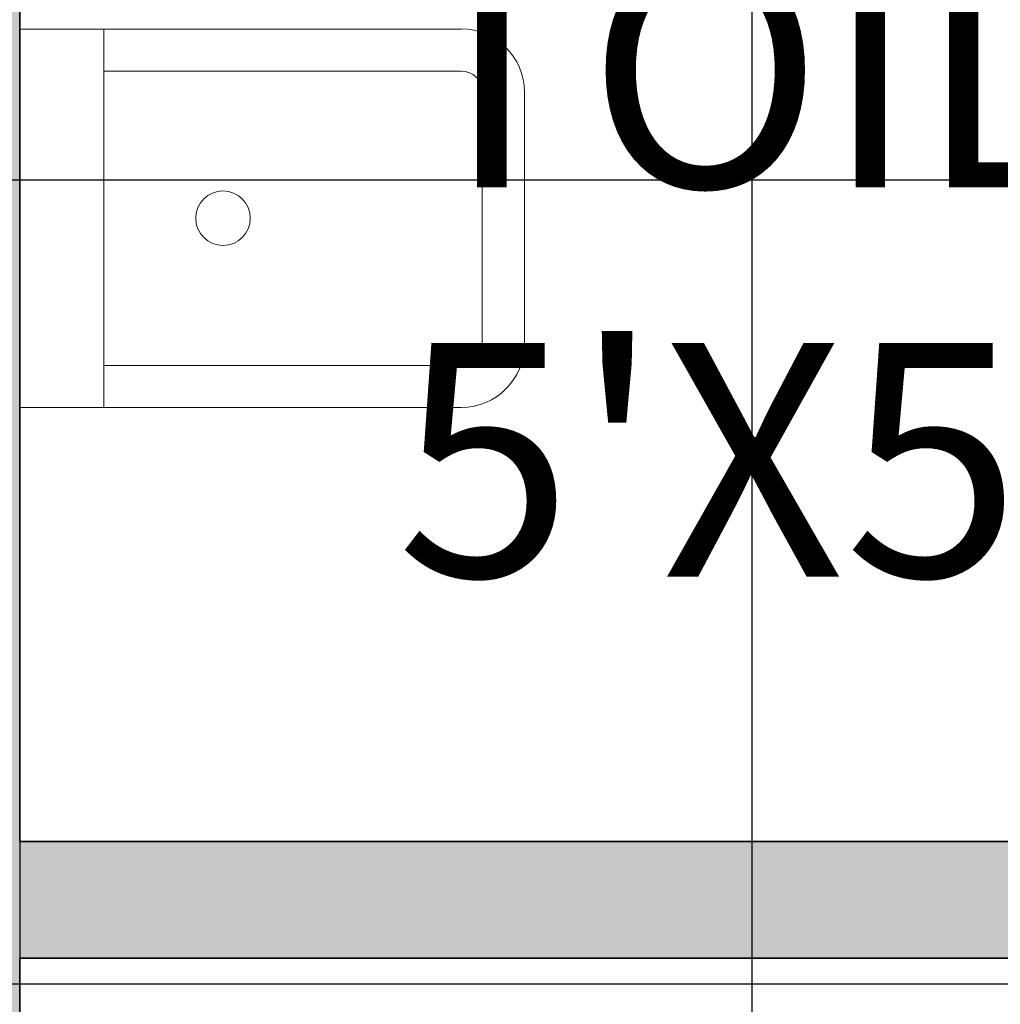
# Model space of a CAD drawing. Units: inches. Extents: x 2696 to 3240, y 1564 to 2310.
# Tile 15 of 76: x 2755 to 2792, y 1852 to 1890. Entities that reach past the tile are written whole.
import ezdxf

# ---------------------------------------------------------------- set-up
doc = ezdxf.new("R2010")
doc.units = ezdxf.units.IN
for name, color, linetype, lineweight in [('A-ANNO-DIMS', 3, 'Continuous', 18), ('A-AREA-IDEN', 7, 'Continuous', 18), ('A-FLOR-FIXT', 8, 'Continuous', 18), ('A-FURN', 251, 'Continuous', 13), ('A-WALL', 7, 'Continuous', 35), ('A-WALL-PATT', 9, 'Continuous', 13)]:
    doc.layers.add(name, color=color, linetype=linetype, lineweight=lineweight)
doc.styles.add('TIMES NEW', font='times.ttf')
doc.styles.add('YQ_DIM', font='SUPEROS.SHX', dxfattribs={"width": 0.8, "bigfont": 'HZDX.SHX'})
doc.dimstyles.new('Siddhuu', dxfattribs={"dimtxt": 6, "dimasz": 2.5, "dimexe": 1.25, "dimexo": 0.625, "dimtad": 1, "dimdec": 1, "dimlunit": 4, "dimtxsty": 'TIMES NEW', "dimcen": 2.5, "dimclrd": 256, "dimclre": 1, "dimclrt": 7, "dimadec": 0, "dimazin": 0, "dimtfac": 1, "dimtdec": 1, "dimtmove": 0, "dimatfit": 3, "dimfxl": 1, "dimtolj": 1, "dimlwd": -1, "dimarcsym": 0})

# ---------------------------------------------------------------- blocks, each defined once
blk = doc.blocks.new('WC')
at = {"layer": 'A-FURN'}
for p, q in [((0, 14.59), (-17.022, 14.59)), ((-3.242, 14.59), (-3.242, 0)), ((-3.242, 12.969), (-17.022, 12.969)), ((-19.454, 2.432), (-19.454, 12.159)), ((-17.833, 2.432), (-17.833, 12.159)), ((-3.242, 1.621), (-17.022, 1.621)), ((0, 0), (-17.022, 0))]:
    blk.add_line(p, q, dxfattribs=at)
blk.add_circle((-7.836, 7.295), 1.051, dxfattribs=at)
for centre, radius, start, end in [((-17.022, 12.159), 2.432, 90, 180), ((-17.022, 12.159), 0.811, 90, 180), ((-17.022, 2.432), 2.432, 180, 270), ((-17.022, 2.432), 0.811, 180, 270)]:
    blk.add_arc(centre, radius, start, end, dxfattribs=at)
blk = doc.blocks.new('*D57')
at = {"layer": 'A-ANNO-DIMS', "color": 1, "lineweight": -2, "transparency": 16777216}
for p, q in [((2754.611, 2018.576), (2754.611, 1568.951)), ((2956.709, 2018.576), (2956.709, 1568.951))]:
    blk.add_line(p, q, dxfattribs=at)
at = {"layer": 'A-ANNO-DIMS', "transparency": 16777216}
blk.add_line((2757.111, 1570.201), (2954.209, 1570.201), dxfattribs=at)
for points in [[(2757.111, 1570.618), (2757.111, 1569.784), (2754.611, 1570.201)], [(2954.209, 1570.618), (2954.209, 1569.784), (2956.709, 1570.201)]]:
    blk.add_solid(points, dxfattribs=at)
at = {"layer": 'Defpoints', "color": 0, "transparency": 16777216}
for p in [(2754.611, 2019.201), (2956.709, 2019.201), (2956.709, 1570.201)]:
    blk.add_point(p, dxfattribs=at)
at = {"layer": 'A-ANNO-DIMS', "color": 7, "transparency": 16777216, "insert": (2855.66, 1573.878), "char_height": 6, "attachment_point": 5, "style": 'TIMES NEW'}
blk.add_mtext('\\A1;16\'-10"', dxfattribs=at)
blk = doc.blocks.new('*D68')
at = {"layer": 'A-ANNO-DIMS', "color": 1, "lineweight": -2, "transparency": 16777216}
for p, q in [((2745.611, 2261.576), (2745.611, 1568.951)), ((2782.834, 2261.576), (2782.834, 1568.951))]:
    blk.add_line(p, q, dxfattribs=at)
at = {"layer": 'A-ANNO-DIMS', "transparency": 16777216}
blk.add_line((2748.111, 1570.201), (2780.334, 1570.201), dxfattribs=at)
for points in [[(2748.111, 1570.618), (2748.111, 1569.784), (2745.611, 1570.201)], [(2780.334, 1570.618), (2780.334, 1569.784), (2782.834, 1570.201)]]:
    blk.add_solid(points, dxfattribs=at)
at = {"layer": 'Defpoints', "color": 0, "transparency": 16777216}
for p in [(2745.611, 2262.201), (2782.834, 2262.201), (2782.834, 1570.201)]:
    blk.add_point(p, dxfattribs=at)
at = {"layer": 'A-ANNO-DIMS', "color": 7, "transparency": 16777216, "insert": (2764.223, 1573.878), "char_height": 6, "attachment_point": 5, "style": 'TIMES NEW'}
blk.add_mtext('\\A1;3\'-1"', dxfattribs=at)
blk = doc.blocks.new('*D79')
at = {"layer": 'A-ANNO-DIMS', "color": 1, "lineweight": -2, "transparency": 16777216}
for p, q in [((3189.986, 1884.201), (2709.361, 1884.201)), ((3189.986, 1853.201), (2709.361, 1853.201))]:
    blk.add_line(p, q, dxfattribs=at)
at = {"layer": 'A-ANNO-DIMS', "transparency": 16777216}
blk.add_line((2710.611, 1881.701), (2710.611, 1855.701), dxfattribs=at)
for points in [[(2710.195, 1881.701), (2711.028, 1881.701), (2710.611, 1884.201)], [(2710.195, 1855.701), (2711.028, 1855.701), (2710.611, 1853.201)]]:
    blk.add_solid(points, dxfattribs=at)
at = {"layer": 'Defpoints', "color": 0, "transparency": 16777216}
for p in [(3190.611, 1884.201), (2710.611, 1853.201), (3190.611, 1853.201)]:
    blk.add_point(p, dxfattribs=at)
at = {"layer": 'A-ANNO-DIMS', "color": 7, "transparency": 16777216, "insert": (2706.926, 1868.701), "char_height": 6, "attachment_point": 5, "rotation": 90, "style": 'TIMES NEW'}
blk.add_mtext('\\A1;2\'-7"', dxfattribs=at)

msp = doc.modelspace()

# ---------------------------------------------------------------- hatches: boundary and pattern name
at = {"layer": 'A-WALL-PATT', "transparency": 33554556}
h = msp.add_hatch(color=256, dxfattribs=at)
h.dxf.hatch_style = 1
h.paths.add_polyline_path([(2879.111, 2253.201), (2905.91, 2253.201), (2905.91, 2262.201), (2841.889, 2262.201), (2841.889, 2253.201), (2870.111, 2253.201), (2870.111, 2176.601), (2965.709, 2176.601), (2965.709, 2206.701), (2973.583, 2206.701), (2973.583, 2215.701), (2965.709, 2215.701), (2965.709, 2262.201), (2929.91, 2262.201), (2929.91, 2253.201), (2956.709, 2253.201), (2956.709, 2185.601), (2879.111, 2185.601)])
h.paths.add_polyline_path([(2782.834, 2262.201), (2745.611, 2262.201), (2745.611, 2228.729), (2754.611, 2228.729), (2754.611, 2253.201), (2782.834, 2253.201)])
h.paths.add_polyline_path([(2754.611, 2136.201), (2965.709, 2136.201), (2965.709, 2145.201), (2879.111, 2145.201), (2879.111, 2147.074), (2877.34, 2147.074), (2870.111, 2147.074), (2870.111, 2145.201), (2754.611, 2145.201), (2754.611, 2169.674), (2745.611, 2169.674), (2745.611, 2000.201), (2754.611, 2000.201), (2754.611, 2019.201), (2849.083, 2019.201), (2849.083, 2023.701), (2841.209, 2023.701), (2841.209, 2051.827), (2836.709, 2051.827), (2836.709, 2023.701), (2754.611, 2023.701), (2754.611, 2091.201), (2836.709, 2091.201), (2836.709, 2087.827), (2841.209, 2087.827), (2841.209, 2095.701), (2754.611, 2095.701)])
h.paths.add_polyline_path([(2965.709, 2136.201), (2956.709, 2136.201), (2956.709, 2023.701), (2885.083, 2023.701), (2885.083, 2019.201), (2956.709, 2019.201), (2956.709, 1950.575), (2965.709, 1950.575), (2965.709, 1980.201), (2973.583, 1980.201), (2973.583, 1989.201), (2965.709, 1989.201)])
h.paths.add_polyline_path([(2754.611, 1906.701), (2880.209, 1906.701), (2884.709, 1906.701), (2956.709, 1906.701), (2956.709, 1792.701), (2944.709, 1792.701), (2944.709, 1783.701), (2956.709, 1783.701), (2956.709, 1740.201), (2884.709, 1740.201), (2884.709, 1783.701), (2896.709, 1783.701), (2896.709, 1792.701), (2884.709, 1792.701), (2884.709, 1846.701), (2880.209, 1846.701), (2880.209, 1740.201), (2754.611, 1740.201), (2754.611, 1777.201), (2745.611, 1777.201), (2745.611, 1692.701), (2754.611, 1692.701), (2754.611, 1731.201), (2956.709, 1731.201), (2956.709, 1723.327), (2965.709, 1723.327), (2965.709, 1884.201), (2973.583, 1884.201), (2973.583, 1893.201), (2965.709, 1893.201), (2965.709, 1914.575), (2956.709, 1914.575), (2956.709, 1911.201), (2754.611, 1911.201), (2754.611, 1930.201), (2745.611, 1930.201), (2745.611, 1817.201), (2754.611, 1817.201), (2754.611, 1854.201), (2826.611, 1854.201), (2826.611, 1868.827), (2822.111, 1868.827), (2822.111, 1858.701), (2754.611, 1858.701)])
h.paths.add_polyline_path([(2965.709, 1656.201), (3008.237, 1656.201), (3008.237, 1665.201), (2965.709, 1665.201), (2965.709, 1693.327), (2956.709, 1693.327), (2956.709, 1686.201), (2934.583, 1686.201), (2934.583, 1681.701), (2956.709, 1681.701), (2956.709, 1614.201), (2896.709, 1614.201), (2896.709, 1681.701), (2904.583, 1681.701), (2904.583, 1686.201), (2892.209, 1686.201), (2892.209, 1614.201), (2858.41, 1614.201), (2858.41, 1605.201), (2965.709, 1605.201)])
h.paths.add_polyline_path([(2788.41, 1614.201), (2754.611, 1614.201), (2754.611, 1652.701), (2745.611, 1652.701), (2745.611, 1605.201), (2788.41, 1605.201)])
h.paths.add_polyline_path([(3199.611, 1633.048), (3190.611, 1633.048), (3190.611, 1614.201), (3082.611, 1614.201), (3082.611, 1665.201), (3070.237, 1665.201), (3070.237, 1656.201), (3078.111, 1656.201), (3078.111, 1605.201), (3199.611, 1605.201)])
h.paths.add_polyline_path([(3199.611, 1702.048), (3190.611, 1702.048), (3190.611, 1699.701), (3106.611, 1699.701), (3106.611, 1747.701), (3190.611, 1747.701), (3190.611, 1752.201), (3082.611, 1752.201), (3082.611, 1760.075), (3078.111, 1760.075), (3078.111, 1747.701), (3102.111, 1747.701), (3102.111, 1699.701), (3078.111, 1699.701), (3078.111, 1695.201), (3190.611, 1695.201), (3190.611, 1676.355), (3199.611, 1676.355)])
h.paths.add_polyline_path([(3199.611, 1783.201), (3190.611, 1783.201), (3190.611, 1745.355), (3199.611, 1745.355)])
h.paths.add_polyline_path([(3082.611, 1884.201), (3190.611, 1884.201), (3190.611, 1853.201), (3199.611, 1853.201), (3199.611, 1901.701), (3190.611, 1901.701), (3190.611, 1893.201), (3005.583, 1893.201), (3005.583, 1891.281), (3005.583, 1884.201), (3078.111, 1884.201), (3078.111, 1792.075), (3082.611, 1792.075)])
h.paths.add_polyline_path([(3199.611, 1994.701), (3190.611, 1994.701), (3190.611, 1989.201), (3073.709, 1989.201), (3073.709, 2034.201), (3069.209, 2034.201), (3069.209, 1989.201), (3005.583, 1989.201), (3005.583, 1980.201), (3190.611, 1980.201), (3190.611, 1971.701), (3199.611, 1971.701)])
h.paths.add_polyline_path([(3199.611, 2155.201), (3190.611, 2155.201), (3190.611, 2064.701), (3199.611, 2064.701)])
h.paths.add_polyline_path([(3190.611, 2074.701), (3106.611, 2074.701), (3106.611, 2122.701), (3190.611, 2122.701), (3190.611, 2127.201), (3082.709, 2127.201), (3082.709, 2135.075), (3073.709, 2135.075), (3073.709, 2122.701), (3102.111, 2122.701), (3102.111, 2074.701), (3069.209, 2074.701), (3069.209, 2070.201), (3190.611, 2070.201)])
h.paths.add_polyline_path([(3082.709, 2253.201), (3190.611, 2253.201), (3190.611, 2225.201), (3199.611, 2225.201), (3199.611, 2262.201), (3073.709, 2262.201), (3073.709, 2215.701), (3035.583, 2215.701), (3035.583, 2206.701), (3073.709, 2206.701), (3073.709, 2171.075), (3082.709, 2171.075)])

# ---------------------------------------------------------------- linework, layer by layer
at = {"layer": 'A-WALL'}
for p, q in [((2754.611, 1858.701), (2754.611, 1906.701)), ((2754.611, 1858.701), (2822.111, 1858.701)), ((2754.611, 1854.201), (2826.611, 1854.201)), ((2754.611, 1817.201), (2754.611, 1854.201))]:
    msp.add_line(p, q, dxfattribs=at)

# ---------------------------------------------------------------- block references
at = {"layer": 'A-FLOR-FIXT', "xscale": -1}
msp.add_blockref('WC', (2754.611, 1875.439), dxfattribs=at)

# ---------------------------------------------------------------- texts
at = {"layer": 'A-AREA-IDEN', "insert": (2769.129, 1892.921), "char_height": 9, "attachment_point": 1, "style": 'YQ_DIM'}
msp.add_mtext_dynamic_manual_height_columns('TOILET\\P5\'X5\'4.5"', width=48.00324, gutter_width=12.5, heights=[0], dxfattribs=at)

# ---------------------------------------------------------------- dimensions: what is measured, and where the dimension line sits
at = {"layer": 'A-ANNO-DIMS'}
for base, p1, p2, picture, middle in [((2782.834, 1570.201), (2745.611, 2262.201), (2782.834, 2262.201), '*D68', (2764.223, 1573.878)), ((2956.709, 1570.201), (2754.611, 2019.201), (2956.709, 2019.201), '*D57', (2855.66, 1573.878))]:
    dim = msp.add_linear_dim(base=base, p1=p1, p2=p2, dimstyle='Siddhuu', override={"dimdec": 1, "dimlfac": 1, "dimrnd": 0, "dimzin": 1, "dimdsep": 46, "dimlunit": 4, "dimfrac": 2}, dxfattribs=at)
    dim.commit()
    dim.dimension.update_dxf_attribs({"geometry": picture, "text_midpoint": middle})
dim = msp.add_linear_dim(base=(2710.611, 1853.201), p1=(3190.611, 1884.201), p2=(3190.611, 1853.201), angle=90, dimstyle='Siddhuu', override={"dimdec": 1, "dimlfac": 1, "dimrnd": 0, "dimzin": 1, "dimdsep": 46, "dimlunit": 4, "dimfrac": 2}, dxfattribs=at)
dim.commit()
dim.dimension.update_dxf_attribs({"geometry": '*D79', "text_midpoint": (2706.926, 1868.701)})

doc.saveas('drawing.dxf')
